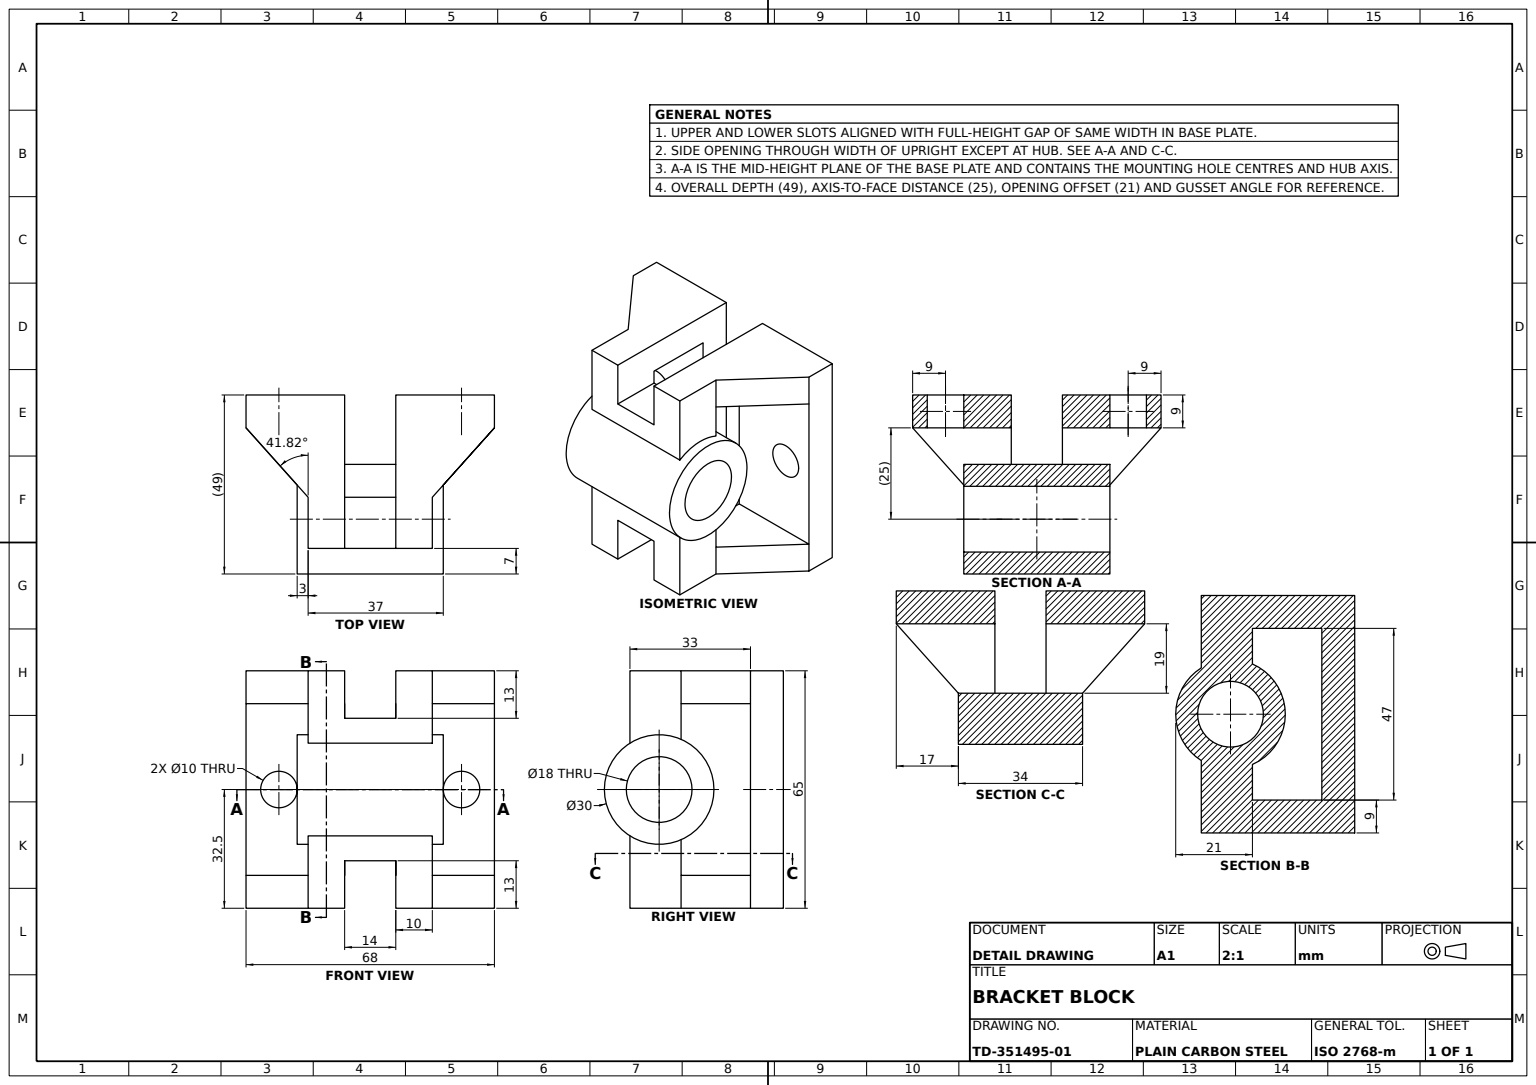
SolidWorks part; units mm, degrees
material "Plain Carbon Steel"
ref_plane "Front Plane" through (0, 0, 0) normal (0, 0, 1) x (1, 0, 0)
ref_plane "Top Plane" through (0, 0, 0) normal (0, 1, 0) x (1, 0, 0)
ref_plane "Right Plane" through (0, 0, 0) normal (1, 0, 0) x (0, 0, -1)
sketch "Base Plate Sketch" plane through (0, 0, 0) normal (0, 0, 1) x (1, 0, 0)
  line L4 (0, 0) -> (68, 0)
  line L5 (68, 0) -> (68, 65)
  line L6 (68, 65) -> (0, 65)
  line L7 (0, 65) -> (0, 0)
  dimension "D2" = 65
  dimension "D1" = 68
  dimension "D3" = 68
extrude "Base Plate 68x65" add sketch "Base Plate Sketch" along normal blind 9
sketch "Upright Block Sketch" plane through (0, 0, 0) normal (0, -1, 0) x (1, 0, 0)
  line L0 (0, 9) -> (68, 9)
  line L8 (34, 42) -> (51, 42)
  line L9 (34, 42) -> (17, 42)
  line L10 (17, 42) -> (17, 28)
  line L11 (17, 28) -> (0, 9)
  line L12 (51, 42) -> (51, 28)
  line L13 (51, 28) -> (68, 9)
  dimension "D1" = 14
  dimension "D2" = 33
  dimension "D3" = 17
  dimension "D4" = 34
  dimension "D6" = 17
  dimension "D7" = 17
extrude "Upright Block" add sketch "Upright Block Sketch" against normal blind 9
sketch "Second Upright Sketch" plane through (0, 65, 0) normal (0, 1, 0) x (1, 0, 0)
  line L0 (34, -42) -> (51, -42)
  line L1 (51, -42) -> (17, -42) construction
  line L2 (51, -42) -> (51, -28)
  line L3 (51, -28) -> (68, -9)
  line L4 (68, -9) -> (0, -9)
  line L5 (0, -9) -> (17, -28)
  line L6 (17, -28) -> (17, -42)
  line L7 (17, -42) -> (34, -42)
extrude "Second Upright Block" add sketch "Second Upright Sketch" against normal blind 9
sketch "Side Web Sketch" plane through (0, 0, 0) normal (0, -1, 0) x (1, 0, 0)
  line L0 (17, 42) -> (17, 28)
  line L1 (17, 28) -> (51, 28)
  line L2 (51, 28) -> (51, 42)
  line L3 (51, 42) -> (17, 42)
extrude "Side Web" add sketch "Side Web Sketch" against normal blind 65
sketch "Upper Slot Sketch" plane through (0, 0, 0) normal (0, -1, 0) x (1, 0, 0)
  line L0 (34, 42) -> (41, 42)
  line L1 (51, 42) -> (17, 42) construction
  line L2 (41, 42) -> (41, 0)
  line L3 (0, 0) -> (68, 0) construction
  line L4 (41, 0) -> (27, 0)
  line L5 (27, 0) -> (27, 42)
  line L6 (27, 42) -> (34, 42)
  dimension "D1" = 7
  dimension "D2" = 14
extrude "Upper Slot 7x14" cut sketch "Upper Slot Sketch" against normal blind 13
sketch "Lower Slot Sketch" plane through (0, 65, 0) normal (0, 1, 0) x (1, 0, 0)
  line L0 (34, -42) -> (41, -42)
  line L1 (17, -42) -> (51, -42) construction
  line L2 (41, -42) -> (41, 0)
  line L3 (41, 0) -> (27, 0)
  line L4 (68, 0) -> (0, 0) construction
  line L5 (27, 0) -> (27, -42)
  line L6 (27, -42) -> (34, -42)
  point P10 (41, -21)
  dimension "D1" = 7
  dimension "D2" = 14
  dimension "D3" = 7
  dimension "D4" = 21
extrude "Lower Slot 7x14" cut sketch "Lower Slot Sketch" against normal blind 13
sketch "Through Channel Sketch" plane through (0, 13, 0) normal (0, -1, 0) x (1, 0, 0)
  line L0 (27, 9) -> (41, 9)
  line L1 (41, 9) -> (41, 0)
  line L2 (41, 0) -> (27, 0)
  line L3 (27, 0) -> (27, 9)
extrude "Through Channel" cut sketch "Through Channel Sketch" against normal blind 65
sketch "Bearing Hub Sketch" plane through (17, 0, 0) normal (-1, 0, 0) x (0, 0, 1)
  line L0 (0, 32.5) -> (34, 32.5)
  line L1 (0, 65) -> (0, 0) construction
  circle A0 centre (34, 32.5) radius 15
  dimension "D2" = 30
  dimension "D1" = 34
extrude "Bearing Hub" add sketch "Bearing Hub Sketch" against normal blind 37
sketch "Hub Collar Sketch Ø30" plane through (17, 0, 0) normal (-1, 0, 0) x (0, 0, 1)
  circle A0 centre (34, 32.5) radius 15
  dimension "D1" = 30
extrude "Hub Collar Ø30" add sketch "Hub Collar Sketch Ø30" along normal blind 3
sketch "Center Bore Sketch Ø18" plane through (14, 0, 0) normal (-1, 0, 0) x (0, 0, 1)
  circle A0 centre (34, 32.5) radius 9
  dimension "D1" = 18
extrude "Center Bore Ø18" cut sketch "Center Bore Sketch Ø18" against normal blind 65
sketch "Side Pocket Sketch" plane through (0, 0, 0) normal (0, 0, -1) x (-1, 0, 0)
  line L0 (-41, 65) -> (-27, 65)
  line L1 (-34, 65) -> (-34, 0)
  line L2 (-34, 32.5) -> (-59, 32.5)
  line L3 (-34, 32.5) -> (-9, 32.5)
  line L5 (-68, 65) -> (-41, 65) construction
  circle A0 centre (-59, 32.5) radius 5
  circle A1 centre (-9, 32.5) radius 5
  dimension "D3" = 10
  dimension "D4" = 10
  dimension "D1" = 25
  dimension "D2" = 25
  dimension "D5" = 32.5
extrude "Side Pocket Cut" cut sketch "Side Pocket Sketch" against normal blind 9
